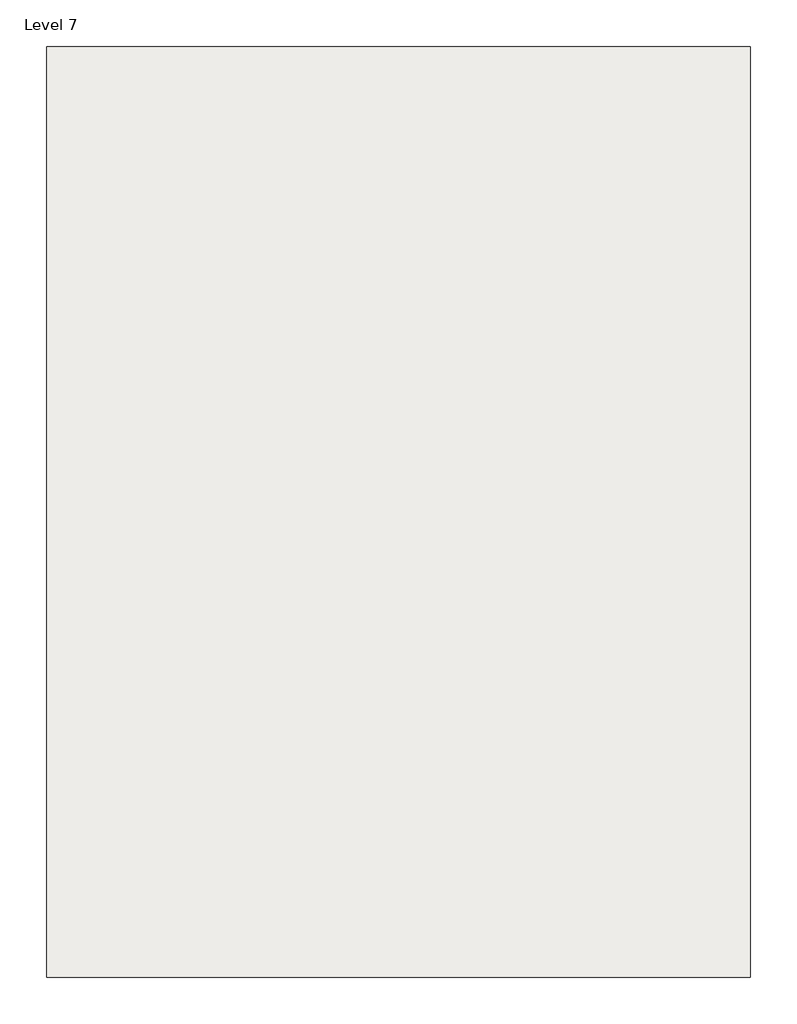
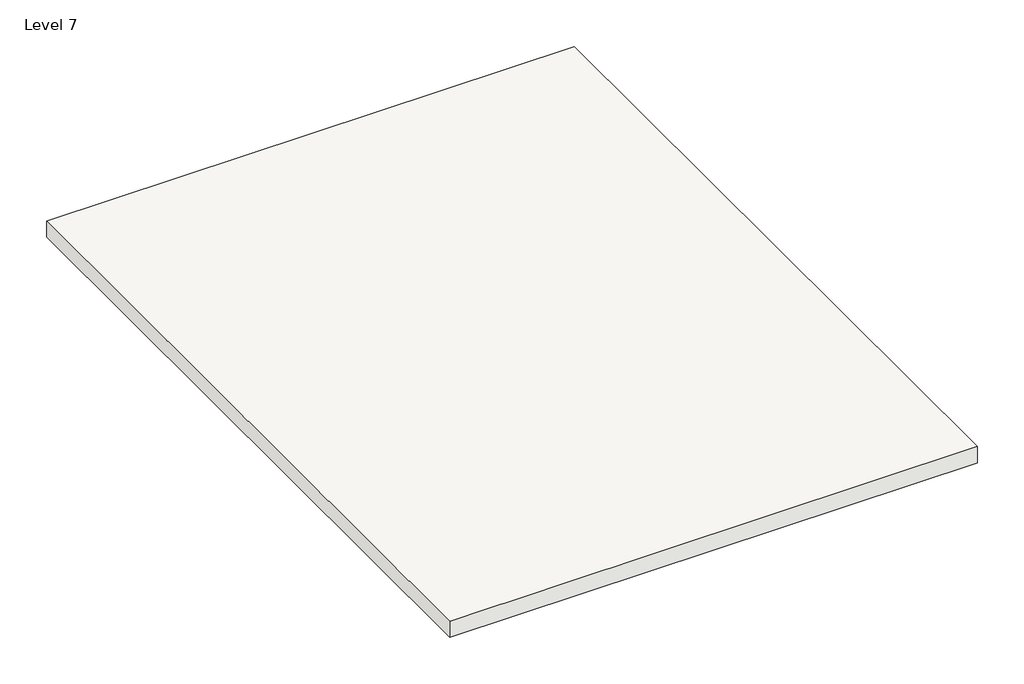
# One storey, incomplete: 1 roof.
"""IFC4 building model written with IfcOpenShell, lengths in millimetres."""

from ifc_helpers import new_model, si_unit, frame, origin, place, context, project, spatial, polyline, outline, extrude, element, save

model = new_model("IFC4")

# Units and contexts
model_context = context("Model", 3, world=origin())
ifc_project = project(units=[si_unit("LENGTHUNIT", "METRE", prefix="MILLI")], contexts=[model_context])

# Site, building, storey
site = spatial("IfcSite", under=ifc_project)
building = spatial("IfcBuilding", under=site)
storey = spatial("IfcBuildingStorey", under=building, Name="Level 7", Elevation=18288.0)

# Roof
placement = place(None, origin())
element("IfcRoof", 1, ObjectType="Generic - 12\"", at=placement, inside=storey, context=model_context, shape_type="SweptSolid", body=[
    extrude(outline(polyline([(406.4, 14579.6), (9855.2, 14579.6), (9855.2, 2082.8), (406.4, 2082.8), (406.4, 14579.6)])), frame((0.0, 0.0, 18288.0), z_axis=(0.0, 0.0, 1.0), x_axis=(1.0, 0.0, 0.0)), (0.0, 0.0, 1.0), 304.8),
])

save(model, "model.ifc")

# Revit data of these elements
# Type "Generic - 12\""
#   Assembly Code = "B1020"
#   Layers, outside or top first: 1' - 0" no material (function 1)
# Element 1 (IfcRoof, "Generic - 12\"")
#   built-in parameter 1001705 = 61 (stored number, unit not read)
#   built-in parameter 1001710 = 33615
#   Phase Created = New Construction
#   Materials on its faces: "Flor_Branco", "Default Roof"
# Materials
#   "Flor_Branco": class "Paint", colour RGB 255 255 255, transparency 0
#   "Default Roof": colour RGB 88 101 114, transparency 0, Cost = 0
